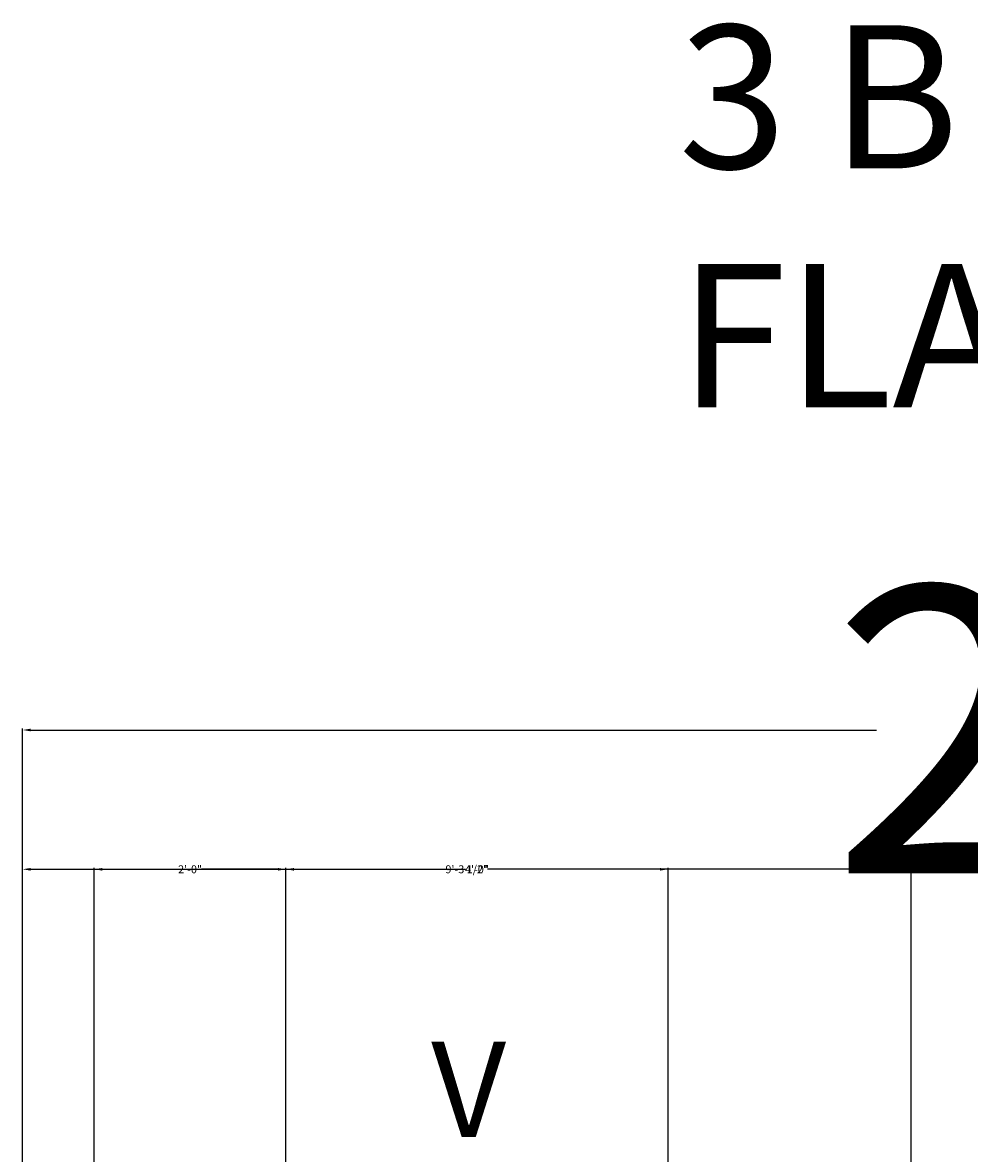
# Model space of a CAD drawing. Units: inches. Extents: x -304 to 580, y 363 to 1149.
# Tile 10 of 11: x -23 to 96, y 1007 to 1149. Entities that reach past the tile are written whole.
import ezdxf

# ---------------------------------------------------------------- set-up
doc = ezdxf.new("R2010")
doc.units = ezdxf.units.IN
doc.header["$MEASUREMENT"] = 0
for name, color, linetype, lineweight in [('A-ANNO-DIMS', 2, 'Continuous', 13), ('A-ANNO-IDEN', 7, 'Continuous', 18), ('A-ANNO-TEXT', 7, 'Continuous', 25)]:
    doc.layers.add(name, color=color, linetype=linetype, lineweight=lineweight)
doc.styles.get("Standard").update_dxf_attribs({"font": 'arial.ttf'})
doc.dimstyles.get("Standard").update_dxf_attribs({"dimtxt": 1, "dimasz": 1, "dimexe": 0.18, "dimexo": 0.0625, "dimgap": 0.09, "dimtad": 0, "dimtih": 1, "dimtoh": 1, "dimdec": 0, "dimzin": 0, "dimdsep": 46, "dimlunit": 3, "dimtxsty": 'Standard', "dimcen": 0.09, "dimadec": 0, "dimazin": 0, "dimtfac": 1, "dimtdec": 0, "dimtofl": 0, "dimtmove": 0, "dimatfit": 3, "dimfxl": 1, "dimtolj": 1, "dimtzin": 0, "dimarcsym": 0})

# ---------------------------------------------------------------- blocks, each defined once
blk = doc.blocks.new('*D2')
at = {"layer": 'A-ANNO-DIMS', "color": 0, "lineweight": -2, "transparency": 16777216}
for p, q in [((-22.57, 1005.01), (-22.57, 1060.38)), ((-21.57, 1060.2), (84.7, 1060.2)), ((315.43, 1060.2), (209.16, 1060.2)), ((316.43, 1005.01), (316.43, 1060.38))]:
    blk.add_line(p, q, dxfattribs=at)
at = {"layer": 'A-ANNO-DIMS', "color": 0, "transparency": 16777216}
for points in [[(-21.57, 1060.37), (-21.57, 1060.04), (-22.57, 1060.2)], [(315.43, 1060.37), (315.43, 1060.04), (316.43, 1060.2)]]:
    blk.add_solid(points, dxfattribs=at)
at = {"layer": 'Defpoints', "color": 0, "transparency": 16777216}
for p in [(316.43, 1060.2), (-22.57, 1004.95), (316.43, 1004.95)]:
    blk.add_point(p, dxfattribs=at)
at = {"layer": 'A-ANNO-DIMS', "color": 0, "transparency": 16777216, "insert": (146.93, 1060.2), "char_height": 1, "attachment_point": 5}
blk.add_mtext('\\A1;{\\H36x;28\'-3"}', dxfattribs=at)
blk = doc.blocks.new('*D34')
at = {"layer": 'A-ANNO-DIMS', "color": 0, "lineweight": -2, "transparency": 16777216}
for p, q in [((10.51, 550.01), (10.51, 1042.88)), ((11.51, 1042.7), (33.07, 1042.7)), ((57.51, 1042.7), (35.95, 1042.7)), ((58.51, 550.01), (58.51, 1042.88))]:
    blk.add_line(p, q, dxfattribs=at)
at = {"layer": 'A-ANNO-DIMS', "color": 0, "transparency": 16777216}
for points in [[(11.51, 1042.86), (11.51, 1042.53), (10.51, 1042.7)], [(57.51, 1042.86), (57.51, 1042.53), (58.51, 1042.7)]]:
    blk.add_solid(points, dxfattribs=at)
at = {"layer": 'Defpoints', "color": 0, "transparency": 16777216}
for p in [(58.51, 1042.7), (10.51, 549.95), (58.51, 549.95)]:
    blk.add_point(p, dxfattribs=at)
at = {"layer": 'A-ANNO-DIMS', "color": 0, "transparency": 16777216, "insert": (34.51, 1042.7), "char_height": 1, "attachment_point": 5}
blk.add_mtext('\\A1;4\'-0"', dxfattribs=at)
blk = doc.blocks.new('*D35')
at = {"layer": 'A-ANNO-DIMS', "color": 0, "lineweight": -2, "transparency": 16777216}
for p, q in [((-13.57, 550.01), (-13.57, 1042.88)), ((-12.57, 1042.7), (-2.96, 1042.7)), ((9.51, 1042.7), (-0.1, 1042.7)), ((10.51, 550.01), (10.51, 1042.88))]:
    blk.add_line(p, q, dxfattribs=at)
at = {"layer": 'A-ANNO-DIMS', "color": 0, "transparency": 16777216}
for points in [[(-12.57, 1042.86), (-12.57, 1042.53), (-13.57, 1042.7)], [(9.51, 1042.86), (9.51, 1042.53), (10.51, 1042.7)]]:
    blk.add_solid(points, dxfattribs=at)
at = {"layer": 'Defpoints', "color": 0, "transparency": 16777216}
for p in [(10.51, 1042.7), (-13.57, 549.95), (10.51, 549.95)]:
    blk.add_point(p, dxfattribs=at)
at = {"layer": 'A-ANNO-DIMS', "color": 0, "transparency": 16777216, "insert": (-1.53, 1042.7), "char_height": 1, "attachment_point": 5}
blk.add_mtext('\\A1;2\'-0"', dxfattribs=at)
blk = doc.blocks.new('*D36')
at = {"layer": 'A-ANNO-DIMS', "color": 0, "lineweight": -2, "transparency": 16777216}
for p, q in [((-22.57, 516.57), (-22.57, 1042.88)), ((-21.57, 1042.7), (30.65, 1042.7)), ((88.04, 1042.7), (35.82, 1042.7)), ((89.04, 516.57), (89.04, 1042.88))]:
    blk.add_line(p, q, dxfattribs=at)
at = {"layer": 'A-ANNO-DIMS', "color": 0, "transparency": 16777216}
for points in [[(-21.57, 1042.86), (-21.57, 1042.53), (-22.57, 1042.7)], [(88.04, 1042.86), (88.04, 1042.53), (89.04, 1042.7)]]:
    blk.add_solid(points, dxfattribs=at)
at = {"layer": 'Defpoints', "color": 0, "transparency": 16777216}
for p in [(89.04, 1042.7), (-22.57, 516.51), (89.04, 516.51)]:
    blk.add_point(p, dxfattribs=at)
at = {"layer": 'A-ANNO-DIMS', "color": 0, "transparency": 16777216, "insert": (33.23, 1042.7), "char_height": 1, "attachment_point": 5}
blk.add_mtext('\\A1;9\'-3 1/2"', dxfattribs=at)

msp = doc.modelspace()

# ---------------------------------------------------------------- texts
at = {"layer": 'A-ANNO-IDEN', "insert": (28.75, 1021.04), "char_height": 12, "attachment_point": 1}
msp.add_mtext_dynamic_manual_height_columns('V', width=10.0311, gutter_width=1, heights=[0], dxfattribs=at)
at = {"layer": 'A-ANNO-TEXT', "insert": (59.82, 1148.78), "char_height": 18, "attachment_point": 1}
msp.add_mtext_dynamic_manual_height_columns('3 BHK RESIDENTIAL FLAT', width=279.8589, gutter_width=1, heights=[0], dxfattribs=at)

# ---------------------------------------------------------------- dimensions: what is measured, and where the dimension line sits
at = {"layer": 'A-ANNO-DIMS'}
dim = msp.add_linear_dim(base=(316.43, 1060.2), p1=(-22.57, 1004.95), p2=(316.43, 1004.95), text='{\\H36x;<>}', dimstyle='Standard', override={"dimclrd": 0, "dimclre": 0, "dimclrt": 0}, dxfattribs=at)
dim.commit()
dim.dimension.update_dxf_attribs({"geometry": '*D2', "text_midpoint": (146.93, 1060.2)})
for base, p1, p2, picture, middle in [((89.04, 1042.7), (-22.57, 516.51), (89.04, 516.51), '*D36', (33.23, 1042.7)), ((10.51, 1042.7), (-13.57, 549.95), (10.51, 549.95), '*D35', (-1.53, 1042.7)), ((58.51, 1042.7), (10.51, 549.95), (58.51, 549.95), '*D34', (34.51, 1042.7))]:
    dim = msp.add_linear_dim(base=base, p1=p1, p2=p2, dimstyle='Standard', override={"dimdec": 1, "dimlfac": 1, "dimrnd": 0, "dimzin": 1, "dimdsep": 46, "dimlunit": 4, "dimfrac": 2}, dxfattribs=at)
    dim.commit()
    dim.dimension.update_dxf_attribs({"geometry": picture, "text_midpoint": middle})

doc.saveas('drawing.dxf')
